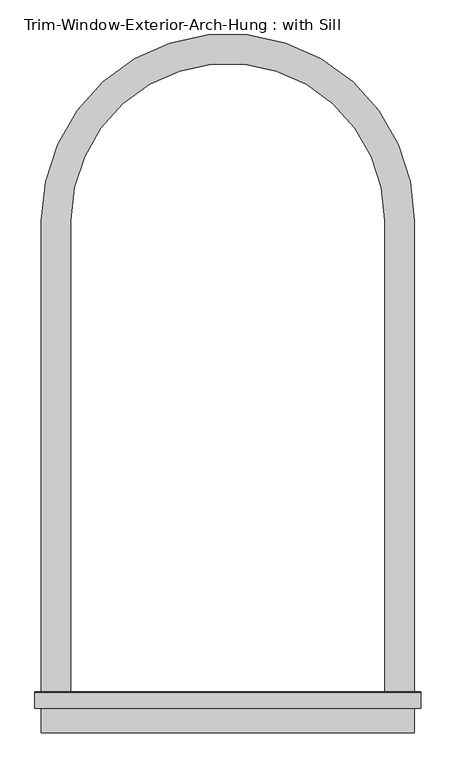
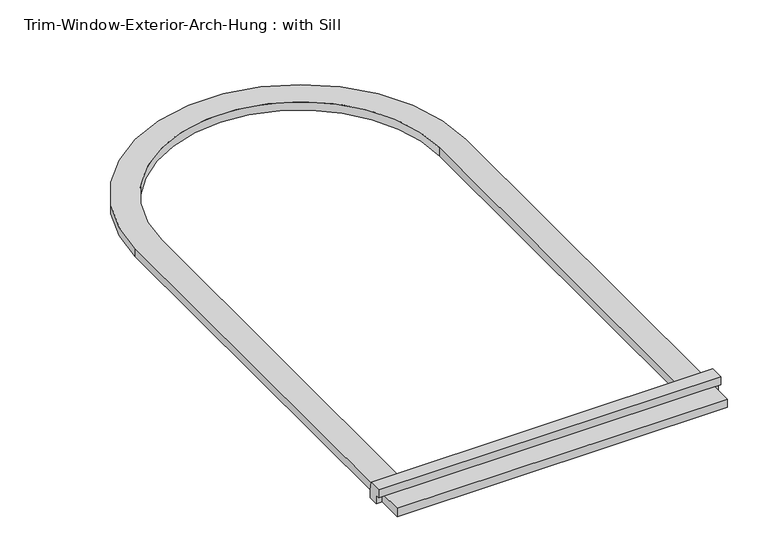
"""IFC4 building model written with IfcOpenShell, lengths in millimetres: proxy geometry, Trim-Window-Exterior-Arch-Hung : with Sill."""

from ifc_helpers import new_model, si_unit, point, frame, frame_2d, origin, origin_with_axes, place, context, project, spatial, polyline, circle_curve, trimmed, segment, composite_curve, outline, extrude, source, transform, mapped, element, save


def trim_window_exterior_arch_hung_with_sill_ae9dfc94(model_context):
    return source(origin(), model_context, "Body", "SweptSolid", [
        extrude(outline(polyline([(361.95, -1241.3823709), (361.95, -1298.5323709), (-361.95, -1298.5323709), (-361.95, -1241.3823709), (361.95, -1241.3823709)])), origin_with_axes(), (0.0, 0.0, 1.0), 19.05),
        extrude(outline(polyline([(-1250.95, 38.1), (-1221.6580645, 38.1), (-1219.2, 19.05), (-1219.2, 0.0), (-1241.3823709, 0.0), (-1241.3823709, 19.05), (-1250.95, 19.05), (-1250.95, 38.1)])), frame((-374.65, 0.0, 0.0), z_axis=(1.0, 0.0, 0.0), x_axis=(0.0, 1.0, 0.0)), (0.0, 0.0, 1.0), 749.3),
        extrude(outline(composite_curve([segment(trimmed(circle_curve(frame_2d((0.0, -304.8)), 361.95), [point((-361.95, -304.8))], [point((361.95, -304.8))], False, "CARTESIAN"), True, "CONTINUOUS"), segment(polyline([(361.95, -304.8), (361.95, -1219.2), (304.8, -1219.2), (304.8, -304.8)]), True, "CONTINUOUS"), segment(trimmed(circle_curve(frame_2d((0.0, -304.8)), 304.8), [point((304.8, -304.8))], [point((-304.8, -304.8))], True, "CARTESIAN"), True, "CONTINUOUS"), segment(polyline([(-304.8, -304.8), (-304.8, -1219.2), (-361.95, -1219.2), (-361.95, -304.8)]), True, "CONTINUOUS")], self_intersect=False)), origin_with_axes(), (0.0, 0.0, 1.0), 19.05),
    ])


if __name__ == "__main__":
    model = new_model("IFC4")
    model_context = context("Model", 3, world=origin())
    ifc_project = project(units=[si_unit("LENGTHUNIT", "METRE", prefix="MILLI")], contexts=[model_context])
    site = spatial("IfcSite", under=ifc_project)
    building = spatial("IfcBuilding", under=site)
    placement = place(None, origin())
    trim_window_exterior_arch_hung_with_sill_shape = trim_window_exterior_arch_hung_with_sill_ae9dfc94(model_context)
    element("IfcBuildingElementProxy", 1, Name="Trim-Window-Exterior-Arch-Hung : with Sill", ObjectType="Trim-Window-Exterior-Arch-Hung : with Sill", at=placement, inside=building, context=model_context, shape_type="MappedRepresentation", body=[
        mapped(trim_window_exterior_arch_hung_with_sill_shape, transform((0.0, 0.0, 0.0), x_axis=(1.0, 0.0, 0.0), y_axis=(0.0, 1.0, 0.0), z_axis=(0.0, 0.0, 1.0))),
    ])
    save(model, "model.ifc")

# Revit data of these elements
# Type "Trim-Window-Exterior-Arch-Hung : with Sill"
#   Trim Width = 0' - 2 1/4"
#   Trim Thickness_Picture Frame = 0' - 1 1/4"
#   Trim Thickness_with Sill = 0' - 0 3/4"
#   Sill Thickness = 0' - 1 1/4"
#   Opening Width [instance default] = 2' - 0"
#   Opening Height [instance default] = 4' - 0"
#   Half Width [instance default] = 1' - 0"
#   Default Elevation = 4' - 0"
#   Sill = yes
#   Picture Frame = no
#   Trim Material [instance default] = none
# Element 1 (IfcBuildingElementProxy, "Trim-Window-Exterior-Arch-Hung : with Sill")
#   Trim Material = Clad - White
#   Materials on its faces: "Clad - White"
# Materials
#   "Clad - White": class "Wood", colour RGB 242 242 238, transparency 0, Cost = 0
